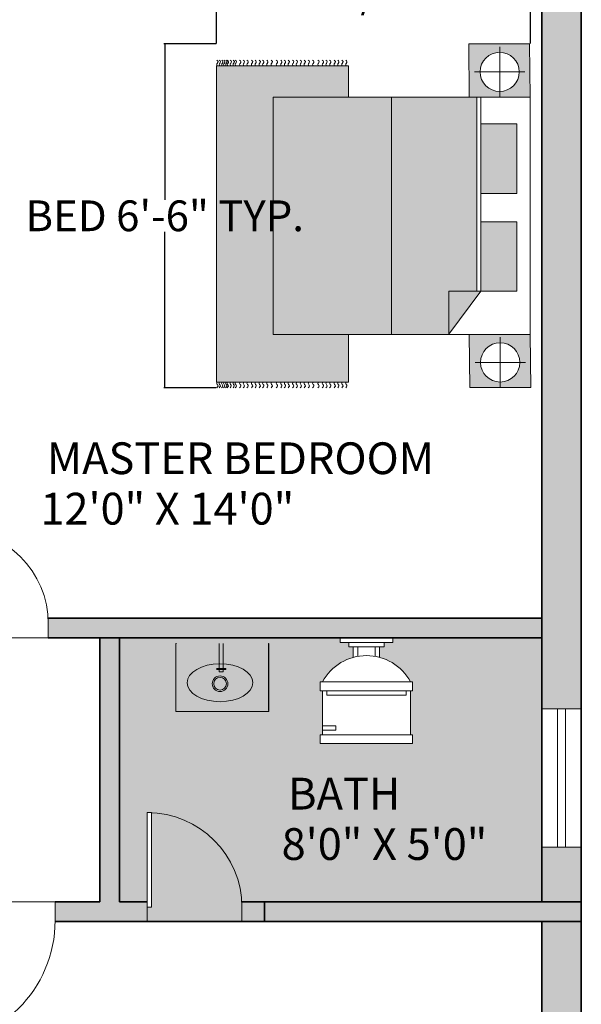
# Model space of a CAD drawing. Units: inches. Extents: x 2167 to 2589, y 1680 to 2489.
# Tile 37 of 38: x 2447 to 2575, y 2143 to 2367. Entities that reach past the tile are written whole.
import ezdxf

# ---------------------------------------------------------------- set-up
doc = ezdxf.new("R2010")
doc.units = ezdxf.units.IN
doc.header["$MEASUREMENT"] = 0
doc.layers.get('0').update_dxf_attribs({"color": 250})
for name, color, linetype, lineweight in [('A-ANNO-DIMS', 2, 'Continuous', 18), ('A-AREA-IDEN', 7, 'Continuous', 18), ('A-DOOR', 4, 'Continuous', 18), ('A-FLOR-FIXT', 8, 'Continuous', 18), ('A-FLOR-TILE-PATT', 252, 'Continuous', 13), ('A-FURN-PATT', 31, 'Continuous', 13), ('A-WALL-PATT', 250, 'Continuous', 13), ('C-PROP', 7, 'Continuous', 35), ('furniture', 34, 'Continuous', 18), ('walls', 7, 'Continuous', 35), ('windows', 141, 'Continuous', 18)]:
    doc.layers.add(name, color=color, linetype=linetype, lineweight=lineweight)
doc.layers.add('A-FLOR-FIXT-PATT', color=7, linetype='Continuous', lineweight=13, true_color=0xebebeb)
doc.styles.get("Standard").update_dxf_attribs({"font": 'arial.ttf'})
doc.dimstyles.get("Standard").update_dxf_attribs({"dimtxt": 7, "dimasz": 0.18, "dimexe": 0.18, "dimexo": 0.0625, "dimgap": 0.09, "dimtad": 0, "dimtih": 1, "dimtoh": 1, "dimdec": 1, "dimzin": 0, "dimdsep": 46, "dimlunit": 3, "dimtxsty": 'Standard', "dimcen": 0.09, "dimadec": 0, "dimazin": 0, "dimtfac": 1, "dimtdec": 1, "dimtofl": 0, "dimtmove": 0, "dimatfit": 3, "dimfxl": 1, "dimtolj": 1, "dimtzin": 0, "dimarcsym": 0})

# ---------------------------------------------------------------- blocks, each defined once
blk = doc.blocks.new('*U2')
for p, q in [((0, 0), (0, -6)), ((40, 0), (40, -6))]:
    blk.add_line(p, q)
blk.add_lwpolyline([(0, 0), (0, 40), (1.75, 40), (1.75, 0)], close=True)
blk.add_arc((0, 0), 40, 0, 90)
blk = doc.blocks.new('*U11')
for p, q in [((-10, 22), (-10, 12)), ((-10, 21), (-7, 21)), ((-7, 21), (-7, 20)), ((10, 12), (10, 22)), ((-7, 20), (-10, 20)), ((10.5, 12), (-10.5, 12)), ((-10.5, 10), (-10.5, 12)), ((9, 13), (-9, 13)), ((-9, 13), (-9, 12)), ((9, 12), (9, 13)), ((10.5, 12), (10.5, 10)), ((10.5, 10), (-10.5, 10)), ((-3, 4.4065), (-3, 2)), ((-2, 2), (-2, 4.1658)), ((2, 4.1658), (2, 2)), ((3, 2), (3, 4.4065)), ((4, 2), (-4, 2)), ((-4, 2), (-4, 1)), ((4, 1), (4, 2))]:
    blk.add_line(p, q)
for points in [[(10.5, 22), (10.5, 24), (-10.5, 24), (-10.5, 22)], [(6, 0), (6, 1), (-6, 1), (-6, 0)]]:
    blk.add_lwpolyline(points, close=True)
blk.add_arc((0, 15.3333), 11.3333, 208.0725, 331.9275)
blk = doc.blocks.new('CARPET')
at = {"layer": 'furniture'}
for p, q in [((-51.53, -98.11), (-51.53, -55.12)), ((-51.53, -55.12), (-41.27, -55.12)), ((36, -55.12), (51.55, -55.12)), ((51.55, -55.12), (51.55, -98.11)), ((51.55, -98.11), (-51.53, -98.11))]:
    blk.add_line(p, q, dxfattribs=at)
for points, knots in [([(-53.37, -55.99), (-53.22, -55.8), (-52.9, -55.41), (-52.34, -55.8), (-51.89, -56.08), (-51.65, -55.91), (-51.53, -55.83)], [0, 0, 0, 0, 0.653278, 1.290138, 1.740457, 2.114451, 2.114451, 2.114451, 2.114451]), ([(-53.37, -57.26), (-53.22, -57.07), (-52.9, -56.67), (-52.34, -57.07), (-51.89, -57.35), (-51.65, -57.17), (-51.53, -57.1)], [0, 0, 0, 0, 0.653278, 1.290138, 1.740457, 2.114451, 2.114451, 2.114451, 2.114451]), ([(53.37, -55.99), (53.22, -55.8), (52.9, -55.41), (52.34, -55.8), (51.89, -56.08), (51.65, -55.91), (51.53, -55.83)], [0, 0, 0, 0, 0.653278, 1.290138, 1.740457, 2.114451, 2.114451, 2.114451, 2.114451]), ([(53.37, -57.26), (53.22, -57.07), (52.9, -56.67), (52.34, -57.07), (51.89, -57.35), (51.65, -57.17), (51.53, -57.1)], [0, 0, 0, 0, 0.653278, 1.290138, 1.740457, 2.114451, 2.114451, 2.114451, 2.114451]), ([(-53.37, -58.59), (-53.22, -58.4), (-52.9, -58.01), (-52.34, -58.4), (-51.89, -58.68), (-51.65, -58.5), (-51.53, -58.43)], [0, 0, 0, 0, 0.653278, 1.290138, 1.740457, 2.114451, 2.114451, 2.114451, 2.114451]), ([(-53.37, -59.78), (-53.22, -59.58), (-52.9, -59.19), (-52.34, -59.58), (-51.89, -59.86), (-51.65, -59.69), (-51.53, -59.61)], [0, 0, 0, 0, 0.653278, 1.290138, 1.740457, 2.114451, 2.114451, 2.114451, 2.114451]), ([(-53.37, -61.22), (-53.22, -61.02), (-52.9, -60.63), (-52.34, -61.02), (-51.89, -61.3), (-51.65, -61.13), (-51.53, -61.05)], [0, 0, 0, 0, 0.653278, 1.290138, 1.740457, 2.114451, 2.114451, 2.114451, 2.114451]), ([(53.37, -58.59), (53.22, -58.4), (52.9, -58.01), (52.34, -58.4), (51.89, -58.68), (51.65, -58.5), (51.53, -58.43)], [0, 0, 0, 0, 0.653278, 1.290138, 1.740457, 2.114451, 2.114451, 2.114451, 2.114451]), ([(53.37, -59.78), (53.22, -59.58), (52.9, -59.19), (52.34, -59.58), (51.89, -59.86), (51.65, -59.69), (51.53, -59.61)], [0, 0, 0, 0, 0.653278, 1.290138, 1.740457, 2.114451, 2.114451, 2.114451, 2.114451]), ([(53.37, -61.22), (53.22, -61.02), (52.9, -60.63), (52.34, -61.02), (51.89, -61.3), (51.65, -61.13), (51.53, -61.05)], [0, 0, 0, 0, 0.653278, 1.290138, 1.740457, 2.114451, 2.114451, 2.114451, 2.114451]), ([(-53.37, -62.44), (-53.22, -62.25), (-52.9, -61.86), (-52.34, -62.25), (-51.89, -62.53), (-51.65, -62.36), (-51.53, -62.28)], [0, 0, 0, 0, 0.653278, 1.290138, 1.740457, 2.114451, 2.114451, 2.114451, 2.114451]), ([(-53.37, -63.63), (-53.22, -63.43), (-52.9, -63.04), (-52.34, -63.43), (-51.89, -63.72), (-51.65, -63.54), (-51.53, -63.46)], [0, 0, 0, 0, 0.653278, 1.290138, 1.740457, 2.114451, 2.114451, 2.114451, 2.114451]), ([(53.37, -62.44), (53.22, -62.25), (52.9, -61.86), (52.34, -62.25), (51.89, -62.53), (51.65, -62.36), (51.53, -62.28)], [0, 0, 0, 0, 0.653278, 1.290138, 1.740457, 2.114451, 2.114451, 2.114451, 2.114451]), ([(53.37, -63.63), (53.22, -63.43), (52.9, -63.04), (52.34, -63.43), (51.89, -63.72), (51.65, -63.54), (51.53, -63.46)], [0, 0, 0, 0, 0.653278, 1.290138, 1.740457, 2.114451, 2.114451, 2.114451, 2.114451]), ([(-53.37, -65.07), (-53.22, -64.87), (-52.9, -64.48), (-52.34, -64.87), (-51.89, -65.15), (-51.65, -64.98), (-51.53, -64.9)], [0, 0, 0, 0, 0.653278, 1.290138, 1.740457, 2.114451, 2.114451, 2.114451, 2.114451]), ([(-53.37, -66.76), (-53.22, -66.56), (-52.9, -66.17), (-52.34, -66.56), (-51.89, -66.84), (-51.65, -66.67), (-51.53, -66.59)], [0, 0, 0, 0, 0.653278, 1.290138, 1.740457, 2.114451, 2.114451, 2.114451, 2.114451]), ([(53.37, -65.07), (53.22, -64.87), (52.9, -64.48), (52.34, -64.87), (51.89, -65.15), (51.65, -64.98), (51.53, -64.9)], [0, 0, 0, 0, 0.653278, 1.290138, 1.740457, 2.114451, 2.114451, 2.114451, 2.114451]), ([(53.37, -66.76), (53.22, -66.56), (52.9, -66.17), (52.34, -66.56), (51.89, -66.84), (51.65, -66.67), (51.53, -66.59)], [0, 0, 0, 0, 0.653278, 1.290138, 1.740457, 2.114451, 2.114451, 2.114451, 2.114451]), ([(-53.37, -68.2), (-53.22, -68), (-52.9, -67.61), (-52.34, -68), (-51.89, -68.28), (-51.65, -68.11), (-51.53, -68.03)], [0, 0, 0, 0, 0.653278, 1.290138, 1.740457, 2.114451, 2.114451, 2.114451, 2.114451]), ([(-53.37, -69.53), (-53.22, -69.33), (-52.9, -68.94), (-52.34, -69.33), (-51.89, -69.61), (-51.65, -69.44), (-51.53, -69.36)], [0, 0, 0, 0, 0.653278, 1.290138, 1.740457, 2.114451, 2.114451, 2.114451, 2.114451]), ([(-53.37, -70.79), (-53.22, -70.6), (-52.9, -70.21), (-52.34, -70.6), (-51.89, -70.88), (-51.65, -70.7), (-51.53, -70.63)], [0, 0, 0, 0, 0.653278, 1.290138, 1.740457, 2.114451, 2.114451, 2.114451, 2.114451]), ([(53.37, -68.2), (53.22, -68), (52.9, -67.61), (52.34, -68), (51.89, -68.28), (51.65, -68.11), (51.53, -68.03)], [0, 0, 0, 0, 0.653278, 1.290138, 1.740457, 2.114451, 2.114451, 2.114451, 2.114451]), ([(53.37, -69.53), (53.22, -69.33), (52.9, -68.94), (52.34, -69.33), (51.89, -69.61), (51.65, -69.44), (51.53, -69.36)], [0, 0, 0, 0, 0.653278, 1.290138, 1.740457, 2.114451, 2.114451, 2.114451, 2.114451]), ([(53.37, -70.79), (53.22, -70.6), (52.9, -70.21), (52.34, -70.6), (51.89, -70.88), (51.65, -70.7), (51.53, -70.63)], [0, 0, 0, 0, 0.653278, 1.290138, 1.740457, 2.114451, 2.114451, 2.114451, 2.114451]), ([(-53.37, -72.12), (-53.22, -71.93), (-52.9, -71.54), (-52.34, -71.93), (-51.89, -72.21), (-51.65, -72.04), (-51.53, -71.96)], [0, 0, 0, 0, 0.653278, 1.290138, 1.740457, 2.114451, 2.114451, 2.114451, 2.114451]), ([(-53.37, -73.31), (-53.22, -73.11), (-52.9, -72.72), (-52.34, -73.11), (-51.89, -73.4), (-51.65, -73.22), (-51.53, -73.14)], [0, 0, 0, 0, 0.653278, 1.290138, 1.740457, 2.114451, 2.114451, 2.114451, 2.114451]), ([(53.37, -72.12), (53.22, -71.93), (52.9, -71.54), (52.34, -71.93), (51.89, -72.21), (51.65, -72.04), (51.53, -71.96)], [0, 0, 0, 0, 0.653278, 1.290138, 1.740457, 2.114451, 2.114451, 2.114451, 2.114451]), ([(53.37, -73.31), (53.22, -73.11), (52.9, -72.72), (52.34, -73.11), (51.89, -73.4), (51.65, -73.22), (51.53, -73.14)], [0, 0, 0, 0, 0.653278, 1.290138, 1.740457, 2.114451, 2.114451, 2.114451, 2.114451]), ([(-53.37, -74.75), (-53.22, -74.55), (-52.9, -74.16), (-52.34, -74.55), (-51.89, -74.83), (-51.65, -74.66), (-51.53, -74.58)], [0, 0, 0, 0, 0.653278, 1.290138, 1.740457, 2.114451, 2.114451, 2.114451, 2.114451]), ([(-53.37, -75.98), (-53.22, -75.78), (-52.9, -75.39), (-52.34, -75.78), (-51.89, -76.06), (-51.65, -75.89), (-51.53, -75.81)], [0, 0, 0, 0, 0.653278, 1.290138, 1.740457, 2.114451, 2.114451, 2.114451, 2.114451]), ([(-53.37, -77.16), (-53.22, -76.96), (-52.9, -76.57), (-52.34, -76.96), (-51.89, -77.25), (-51.65, -77.07), (-51.53, -76.99)], [0, 0, 0, 0, 0.653278, 1.290138, 1.740457, 2.114451, 2.114451, 2.114451, 2.114451]), ([(53.37, -74.75), (53.22, -74.55), (52.9, -74.16), (52.34, -74.55), (51.89, -74.83), (51.65, -74.66), (51.53, -74.58)], [0, 0, 0, 0, 0.653278, 1.290138, 1.740457, 2.114451, 2.114451, 2.114451, 2.114451]), ([(53.37, -75.98), (53.22, -75.78), (52.9, -75.39), (52.34, -75.78), (51.89, -76.06), (51.65, -75.89), (51.53, -75.81)], [0, 0, 0, 0, 0.653278, 1.290138, 1.740457, 2.114451, 2.114451, 2.114451, 2.114451]), ([(53.37, -77.16), (53.22, -76.96), (52.9, -76.57), (52.34, -76.96), (51.89, -77.25), (51.65, -77.07), (51.53, -76.99)], [0, 0, 0, 0, 0.653278, 1.290138, 1.740457, 2.114451, 2.114451, 2.114451, 2.114451]), ([(-53.37, -78.6), (-53.22, -78.4), (-52.9, -78.01), (-52.34, -78.4), (-51.89, -78.68), (-51.65, -78.51), (-51.53, -78.43)], [0, 0, 0, 0, 0.653278, 1.290138, 1.740457, 2.114451, 2.114451, 2.114451, 2.114451]), ([(-53.37, -80.29), (-53.22, -80.09), (-52.9, -79.7), (-52.34, -80.09), (-51.89, -80.37), (-51.65, -80.2), (-51.53, -80.12)], [0, 0, 0, 0, 0.653278, 1.290138, 1.740457, 2.114451, 2.114451, 2.114451, 2.114451]), ([(53.37, -78.6), (53.22, -78.4), (52.9, -78.01), (52.34, -78.4), (51.89, -78.68), (51.65, -78.51), (51.53, -78.43)], [0, 0, 0, 0, 0.653278, 1.290138, 1.740457, 2.114451, 2.114451, 2.114451, 2.114451]), ([(53.37, -80.29), (53.22, -80.09), (52.9, -79.7), (52.34, -80.09), (51.89, -80.37), (51.65, -80.2), (51.53, -80.12)], [0, 0, 0, 0, 0.653278, 1.290138, 1.740457, 2.114451, 2.114451, 2.114451, 2.114451]), ([(-53.37, -81.73), (-53.22, -81.53), (-52.9, -81.14), (-52.34, -81.53), (-51.89, -81.81), (-51.65, -81.64), (-51.53, -81.56)], [0, 0, 0, 0, 0.653278, 1.290138, 1.740457, 2.114451, 2.114451, 2.114451, 2.114451]), ([(-53.37, -83.06), (-53.22, -82.86), (-52.9, -82.47), (-52.34, -82.86), (-51.89, -83.14), (-51.65, -82.97), (-51.53, -82.89)], [0, 0, 0, 0, 0.653278, 1.290138, 1.740457, 2.114451, 2.114451, 2.114451, 2.114451]), ([(53.37, -81.73), (53.22, -81.53), (52.9, -81.14), (52.34, -81.53), (51.89, -81.81), (51.65, -81.64), (51.53, -81.56)], [0, 0, 0, 0, 0.653278, 1.290138, 1.740457, 2.114451, 2.114451, 2.114451, 2.114451]), ([(53.37, -83.06), (53.22, -82.86), (52.9, -82.47), (52.34, -82.86), (51.89, -83.14), (51.65, -82.97), (51.53, -82.89)], [0, 0, 0, 0, 0.653278, 1.290138, 1.740457, 2.114451, 2.114451, 2.114451, 2.114451]), ([(-53.37, -84.18), (-53.22, -83.99), (-52.9, -83.6), (-52.34, -83.99), (-51.89, -84.27), (-51.65, -84.09), (-51.53, -84.02)], [0, 0, 0, 0, 0.653278, 1.290138, 1.740457, 2.114451, 2.114451, 2.114451, 2.114451]), ([(-53.37, -85.51), (-53.22, -85.32), (-52.9, -84.93), (-52.34, -85.32), (-51.89, -85.6), (-51.65, -85.42), (-51.53, -85.35)], [0, 0, 0, 0, 0.653278, 1.290138, 1.740457, 2.114451, 2.114451, 2.114451, 2.114451]), ([(-53.37, -86.7), (-53.22, -86.5), (-52.9, -86.11), (-52.34, -86.5), (-51.89, -86.78), (-51.65, -86.61), (-51.53, -86.53)], [0, 0, 0, 0, 0.653278, 1.290138, 1.740457, 2.114451, 2.114451, 2.114451, 2.114451]), ([(53.37, -84.18), (53.22, -83.99), (52.9, -83.6), (52.34, -83.99), (51.89, -84.27), (51.65, -84.09), (51.53, -84.02)], [0, 0, 0, 0, 0.653278, 1.290138, 1.740457, 2.114451, 2.114451, 2.114451, 2.114451]), ([(53.37, -85.51), (53.22, -85.32), (52.9, -84.93), (52.34, -85.32), (51.89, -85.6), (51.65, -85.42), (51.53, -85.35)], [0, 0, 0, 0, 0.653278, 1.290138, 1.740457, 2.114451, 2.114451, 2.114451, 2.114451]), ([(53.37, -86.7), (53.22, -86.5), (52.9, -86.11), (52.34, -86.5), (51.89, -86.78), (51.65, -86.61), (51.53, -86.53)], [0, 0, 0, 0, 0.653278, 1.290138, 1.740457, 2.114451, 2.114451, 2.114451, 2.114451]), ([(-53.37, -88.14), (-53.22, -87.94), (-52.9, -87.55), (-52.34, -87.94), (-51.89, -88.22), (-51.65, -88.05), (-51.53, -87.97)], [0, 0, 0, 0, 0.653278, 1.290138, 1.740457, 2.114451, 2.114451, 2.114451, 2.114451]), ([(-53.37, -89.36), (-53.22, -89.17), (-52.9, -88.78), (-52.34, -89.17), (-51.89, -89.45), (-51.65, -89.28), (-51.53, -89.2)], [0, 0, 0, 0, 0.653278, 1.290138, 1.740457, 2.114451, 2.114451, 2.114451, 2.114451]), ([(53.37, -88.14), (53.22, -87.94), (52.9, -87.55), (52.34, -87.94), (51.89, -88.22), (51.65, -88.05), (51.53, -87.97)], [0, 0, 0, 0, 0.653278, 1.290138, 1.740457, 2.114451, 2.114451, 2.114451, 2.114451]), ([(53.37, -89.36), (53.22, -89.17), (52.9, -88.78), (52.34, -89.17), (51.89, -89.45), (51.65, -89.28), (51.53, -89.2)], [0, 0, 0, 0, 0.653278, 1.290138, 1.740457, 2.114451, 2.114451, 2.114451, 2.114451]), ([(-53.37, -90.55), (-53.22, -90.35), (-52.9, -89.96), (-52.34, -90.35), (-51.89, -90.64), (-51.65, -90.46), (-51.53, -90.38)], [0, 0, 0, 0, 0.653278, 1.290138, 1.740457, 2.114451, 2.114451, 2.114451, 2.114451]), ([(-53.37, -91.99), (-53.22, -91.79), (-52.9, -91.4), (-52.34, -91.79), (-51.89, -92.07), (-51.65, -91.9), (-51.53, -91.82)], [0, 0, 0, 0, 0.653278, 1.290138, 1.740457, 2.114451, 2.114451, 2.114451, 2.114451]), ([(-53.37, -92.69), (-53.22, -92.48), (-52.9, -92.08), (-52.35, -92.49), (-51.89, -92.77), (-51.65, -92.6), (-51.53, -92.52)], [0, 0, 0, 0, 0.663904, 1.307406, 1.757725, 2.131719, 2.131719, 2.131719, 2.131719]), ([(53.37, -90.55), (53.22, -90.35), (52.9, -89.96), (52.34, -90.35), (51.9, -90.63), (51.66, -90.47), (51.55, -90.4)], [0, 0, 0, 0, 0.653278, 1.290138, 1.740457, 2.0926, 2.0926, 2.0926, 2.0926]), ([(53.37, -91.99), (53.22, -91.79), (52.9, -91.4), (52.34, -91.79), (51.9, -92.07), (51.66, -91.91), (51.55, -91.83)], [0, 0, 0, 0, 0.653278, 1.290138, 1.740457, 2.0926, 2.0926, 2.0926, 2.0926]), ([(53.37, -92.69), (53.22, -92.49), (52.9, -92.09), (52.34, -92.49), (51.9, -92.77), (51.66, -92.61), (51.55, -92.53)], [0, 0, 0, 0, 0.656792, 1.295826, 1.746145, 2.098292, 2.098292, 2.098292, 2.098292]), ([(-53.37, -93.61), (-53.22, -93.42), (-52.9, -93.03), (-52.34, -93.42), (-51.89, -93.7), (-51.65, -93.52), (-51.53, -93.45)], [0, 0, 0, 0, 0.653278, 1.290138, 1.740457, 2.114451, 2.114451, 2.114451, 2.114451]), ([(-53.37, -94.55), (-53.22, -94.35), (-52.9, -93.96), (-52.34, -94.35), (-51.89, -94.63), (-51.65, -94.46), (-51.53, -94.38)], [0, 0, 0, 0, 0.653278, 1.290138, 1.740457, 2.114451, 2.114451, 2.114451, 2.114451]), ([(-53.37, -95.05), (-53.22, -94.85), (-52.9, -94.46), (-52.34, -94.85), (-51.89, -95.14), (-51.65, -94.96), (-51.53, -94.88)], [0, 0, 0, 0, 0.653278, 1.290138, 1.740457, 2.114451, 2.114451, 2.114451, 2.114451]), ([(-53.37, -95.73), (-53.22, -95.54), (-52.9, -95.15), (-52.34, -95.54), (-51.89, -95.82), (-51.65, -95.65), (-51.53, -95.57)], [0, 0, 0, 0, 0.653278, 1.290138, 1.740457, 2.114451, 2.114451, 2.114451, 2.114451]), ([(-53.37, -96.38), (-53.22, -96.18), (-52.9, -95.79), (-52.34, -96.18), (-51.89, -96.47), (-51.65, -96.29), (-51.53, -96.21)], [0, 0, 0, 0, 0.653278, 1.290138, 1.740457, 2.114451, 2.114451, 2.114451, 2.114451]), ([(53.37, -95.78), (53.22, -95.58), (52.9, -95.19), (52.34, -95.58), (51.89, -95.86), (51.65, -95.69), (51.53, -95.61)], [0, 0, 0, 0, 0.653278, 1.290138, 1.740457, 2.114451, 2.114451, 2.114451, 2.114451]), ([(53.37, -96.43), (53.22, -96.23), (52.9, -95.84), (52.34, -96.23), (51.89, -96.51), (51.65, -96.34), (51.53, -96.26)], [0, 0, 0, 0, 0.653278, 1.290138, 1.740457, 2.114451, 2.114451, 2.114451, 2.114451]), ([(53.37, -93.66), (53.22, -93.46), (52.9, -93.07), (52.34, -93.46), (51.9, -93.74), (51.66, -93.58), (51.55, -93.5)], [0, 0, 0, 0, 0.653278, 1.290138, 1.740457, 2.0926, 2.0926, 2.0926, 2.0926]), ([(53.37, -94.59), (53.22, -94.4), (52.9, -94.01), (52.34, -94.4), (51.9, -94.68), (51.66, -94.51), (51.55, -94.44)], [0, 0, 0, 0, 0.653278, 1.290138, 1.740457, 2.0926, 2.0926, 2.0926, 2.0926]), ([(53.37, -95.1), (53.22, -94.9), (52.9, -94.51), (52.34, -94.9), (51.9, -95.18), (51.66, -95.02), (51.55, -94.94)], [0, 0, 0, 0, 0.653278, 1.290138, 1.740457, 2.0926, 2.0926, 2.0926, 2.0926]), ([(-53.37, -97.17), (-53.22, -96.98), (-52.9, -96.59), (-52.34, -96.98), (-51.89, -97.26), (-51.65, -97.08), (-51.53, -97.01)], [0, 0, 0, 0, 0.653278, 1.290138, 1.740457, 2.114451, 2.114451, 2.114451, 2.114451]), ([(-53.37, -97.99), (-53.22, -97.79), (-52.9, -97.4), (-52.34, -97.79), (-51.89, -98.08), (-51.65, -97.9), (-51.53, -97.82)], [0, 0, 0, 0, 0.653278, 1.290138, 1.740457, 2.114451, 2.114451, 2.114451, 2.114451]), ([(53.37, -97.22), (53.22, -97.02), (52.9, -96.63), (52.34, -97.02), (51.89, -97.3), (51.65, -97.13), (51.53, -97.05)], [0, 0, 0, 0, 0.653278, 1.290138, 1.740457, 2.114451, 2.114451, 2.114451, 2.114451]), ([(53.37, -97.99), (53.22, -97.79), (52.9, -97.4), (52.34, -97.79), (51.89, -98.08), (51.65, -97.9), (51.53, -97.82)], [0, 0, 0, 0, 0.653278, 1.290138, 1.740457, 2.114451, 2.114451, 2.114451, 2.114451])]:
    blk.add_open_spline(points, degree=3, knots=knots, dxfattribs=at)
blk = doc.blocks.new('A$C58D270C6')
at = {"layer": 'furniture'}
for p, q in [((9.09, 124.13), (9.09, 108.87)), ((1.46, 116.5), (16.73, 116.5)), ((14.97, 94.84), (24.62, 107.92)), ((24.62, 94.93), (24.62, 107.92)), ((42.08, 108), (42.08, 36)), ((14.97, 94.93), (24.62, 94.93)), ((14.97, 94.84), (14.97, 36)), ((16.22, 94.93), (16.22, 36)), ((9.25, 36), (9.25, 20.74)), ((1.62, 28.37), (16.88, 28.37))]:
    blk.add_line(p, q, dxfattribs=at)
for points in [[(18.5, 108), (18.34, 124.13), (-0.16, 124.13), (0, 108)], [(0, 108), (77.91, 108), (77.91, 36), (0, 36)], [(4.09, 94.93), (14.97, 94.93), (14.97, 73.83), (4.09, 73.83)], [(4.09, 65.23), (14.97, 65.23), (14.97, 44.13), (4.09, 44.13)], [(18.65, 19.87), (18.5, 36), (0, 36), (0.16, 19.87)]]:
    blk.add_lwpolyline(points, close=True, dxfattribs=at)
for centre in [(9.09, 116.5), (9.25, 28.37)]:
    blk.add_circle(centre, 5.95, dxfattribs=at)
at = {"layer": 'furniture', "xscale": 0.9312884925094044, "yscale": 0.9312884925094044, "zscale": 0.9312884925094044, "rotation": 90}
blk.add_blockref('CARPET', (3.79, 74.47), dxfattribs=at)
blk = doc.blocks.new('LAV-OVAL-WITH-TAP')
for p, q in [((6.14, 5.63), (6.14, 5.92)), ((6.14, 5.92), (8.26, 5.92)), ((8.26, 5.63), (6.14, 5.63)), ((7.69, 6.42), (6.74, 6.42)), ((6.74, 6.42), (6.74, 0)), ((7.69, 6.42), (7.69, 0))]:
    blk.add_line(p, q)
for radius in [1.79, 1.79, 1.43, 1.43, 1.43, 1.43]:
    blk.add_circle((7.46, 9.13), radius)
blk.add_ellipse((7.48, 8.9), major_axis=(7.48, 0.02), ratio=0.576535)
blk = doc.blocks.new('*D43')
at = {"layer": 'A-ANNO-DIMS', "color": 0, "lineweight": -2, "transparency": 16777216}
for p, q in [((2491.99, 2361.37), (2480.13, 2361.37)), ((2480.31, 2361.19), (2480.31, 2325.91)), ((2480.31, 2283.31), (2480.31, 2318.59)), ((2491.99, 2283.13), (2480.13, 2283.13))]:
    blk.add_line(p, q, dxfattribs=at)
at = {"layer": 'A-ANNO-DIMS', "color": 0, "transparency": 16777216}
for points in [[(2480.28, 2361.19), (2480.34, 2361.19), (2480.31, 2361.37)], [(2480.28, 2283.31), (2480.34, 2283.31), (2480.31, 2283.13)]]:
    blk.add_solid(points, dxfattribs=at)
at = {"layer": 'Defpoints', "color": 0, "transparency": 16777216}
for p in [(2492.05, 2361.37), (2480.31, 2283.13), (2492.05, 2283.13)]:
    blk.add_point(p, dxfattribs=at)
at = {"layer": 'A-ANNO-DIMS', "color": 0, "transparency": 16777216, "insert": (2480.31, 2322.25), "char_height": 7, "attachment_point": 5}
blk.add_mtext('\\A1;BED 6\'-6" TYP.', dxfattribs=at)
blk = doc.blocks.new('*D44')
at = {"layer": 'A-ANNO-DIMS', "color": 0, "lineweight": -2, "transparency": 16777216}
for p, q in [((2492.05, 2361.43), (2492.05, 2373.28)), ((2492.23, 2373.1), (2495.49, 2373.1)), ((2563.35, 2373.1), (2560.09, 2373.1)), ((2563.53, 2361.43), (2563.53, 2373.28))]:
    blk.add_line(p, q, dxfattribs=at)
at = {"layer": 'A-ANNO-DIMS', "color": 0, "transparency": 16777216}
for points in [[(2492.23, 2373.13), (2492.23, 2373.07), (2492.05, 2373.1)], [(2563.35, 2373.13), (2563.35, 2373.07), (2563.53, 2373.1)]]:
    blk.add_solid(points, dxfattribs=at)
at = {"layer": 'Defpoints', "color": 0, "transparency": 16777216}
for p in [(2492.05, 2373.1), (2492.05, 2361.37), (2563.53, 2361.37)]:
    blk.add_point(p, dxfattribs=at)
at = {"layer": 'A-ANNO-DIMS', "color": 0, "transparency": 16777216, "insert": (2527.79, 2373.1), "char_height": 7, "attachment_point": 5}
blk.add_mtext('\\A1;5\'-11 1/2" TYP.', dxfattribs=at)

msp = doc.modelspace()

# ---------------------------------------------------------------- hatches: boundary and pattern name
at = {"layer": 'A-FLOR-FIXT-PATT'}
h = msp.add_hatch(color=256, dxfattribs=at)
h.dxf.hatch_style = 1
edge = h.paths.add_edge_path()
edge.add_line((2483, 2209.66), (2503.9, 2209.66))
edge.add_line((2503.9, 2209.66), (2503.9, 2224.91))
edge.add_line((2503.9, 2224.91), (2493.61, 2224.91))
edge.add_line((2493.61, 2224.91), (2493.61, 2220.31))
edge.add_ellipse((2492.87, 2216.02), major_axis=(-7.48, -0.02), ratio=0.576535, start_angle=272.6137, end_angle=620.1108, ccw=False)
edge.add_line((2492.66, 2220.33), (2492.66, 2224.91))
edge.add_line((2492.66, 2224.91), (2483, 2224.91))
edge.add_line((2483, 2224.91), (2483, 2209.66))
h = msp.add_hatch(color=256, dxfattribs=at)
h.dxf.hatch_style = 1
edge = h.paths.add_edge_path()
edge.add_ellipse((2492.87, 2216.02), major_axis=(-7.48, -0.02), ratio=0.576535, start_angle=272.6137, end_angle=260.1108)
edge.add_line((2493.61, 2220.31), (2493.61, 2219.29))
edge.add_line((2493.61, 2219.29), (2494.21, 2219.29))
edge.add_line((2494.21, 2219.29), (2494.21, 2218.99))
edge.add_line((2494.21, 2218.99), (2493.61, 2218.99))
edge.add_line((2493.61, 2218.99), (2493.61, 2218.49))
edge.add_line((2493.61, 2218.49), (2492.66, 2218.49))
edge.add_line((2492.66, 2218.49), (2492.66, 2220.33))
h.paths.add_polyline_path([(2491.1, 2215.78, -1), (2494.67, 2215.78, -1)], flags=16)
h.paths.add_polyline_path([(2494.31, 2215.78, -1), (2491.46, 2215.78, -1)], flags=0)
h.paths.add_polyline_path([(2491.46, 2215.78, 1), (2494.31, 2215.78, 1)], flags=0)
edge = h.paths.add_edge_path()
edge.add_line((2492.66, 2219.29), (2493.61, 2219.29))
edge.add_line((2493.61, 2219.29), (2493.61, 2220.31))
edge.add_ellipse((2492.87, 2216.02), major_axis=(-7.48, -0.02), ratio=0.576535, start_angle=260.1108, end_angle=272.6137)
edge.add_line((2492.66, 2220.33), (2492.66, 2219.29))
h.paths.add_polyline_path([(2492.66, 2218.49), (2493.61, 2218.49), (2493.61, 2218.99), (2492.66, 2218.99)], flags=17)
h.paths.add_polyline_path([(2492.66, 2218.99), (2493.61, 2218.99), (2493.61, 2219.29), (2492.66, 2219.29)], flags=17)
h.paths.add_polyline_path([(2493.61, 2218.99), (2494.21, 2218.99), (2494.21, 2219.29), (2493.61, 2219.29)], flags=17)
edge = h.paths.add_edge_path()
edge.add_ellipse((2492.87, 2216.02), major_axis=(-7.48, -0.02), ratio=0.576535, start_angle=260.1108, end_angle=272.6137, ccw=False)
edge.add_line((2493.61, 2220.31), (2493.61, 2224.91))
edge.add_line((2493.61, 2224.91), (2492.66, 2224.91))
edge.add_line((2492.66, 2224.91), (2492.66, 2220.33))
h = msp.add_hatch(color=256, dxfattribs=at)
h.dxf.hatch_style = 1
h.paths.add_polyline_path([(2494.31, 2215.78, 1), (2491.46, 2215.78, 1)], flags=0)
h.paths.add_polyline_path([(2494.67, 2215.78, 1), (2491.1, 2215.78, 1)])
h.paths.add_polyline_path([(2494.31, 2215.78, -1), (2491.46, 2215.78, -1)], flags=16)
h = msp.add_hatch(color=256, dxfattribs=at)
h.dxf.hatch_style = 1
h.paths.add_polyline_path([(2494.31, 2215.78, 1), (2491.46, 2215.78, 1)])
at = {"layer": 'A-FLOR-TILE-PATT'}
h = msp.add_hatch(dxfattribs=at)
h.set_pattern_fill('ANGLE', color=256, scale=5)
h.set_pattern_definition([(0, (0, 0), (0, 1.375), [1, -0.375]), (90, (0, 0), (-1.375, 1e-16), [1, -0.375])])
h.paths.add_polyline_path([(2566.05, 2226.19), (2532.19, 2226.19), (2532.19, 2225.19), (2530.19, 2225.19), (2530.19, 2224.19), (2529.19, 2224.19), (2529.19, 2221.79, -0.206081), (2536.19, 2216.19), (2536.69, 2216.19), (2536.69, 2214.19), (2536.19, 2214.19), (2536.19, 2204.19), (2536.69, 2204.19), (2536.69, 2202.19), (2515.69, 2202.19), (2515.69, 2204.19), (2516.19, 2204.19), (2516.19, 2214.19), (2515.69, 2214.19), (2515.69, 2216.19), (2516.19, 2216.19, -0.206081), (2523.19, 2221.79), (2523.19, 2224.19), (2522.19, 2224.19), (2522.19, 2225.19), (2520.19, 2225.19), (2520.19, 2226.19), (2470.05, 2226.19), (2470.05, 2166.19), (2476.35, 2166.19), (2476.35, 2186.45), (2477.29, 2186.45), (2477.29, 2186.43, -0.38441), (2497.84, 2166.19), (2566.05, 2166.19)])
h.paths.add_polyline_path([(2504.02, 2209.46), (2504.02, 2224.91), (2503.9, 2224.91), (2503.9, 2209.66)], flags=16)
edge = h.paths.add_edge_path(flags=16)
edge.add_ellipse((2492.87, 2216.02), major_axis=(-7.48, -0.02), ratio=0.576535, start_angle=272.6137, end_angle=620.1108, ccw=False)
edge.add_ellipse((2492.87, 2216.02), major_axis=(-7.48, -0.02), ratio=0.576535, start_angle=260.1108, end_angle=272.6137, ccw=False)
h.paths.add_polyline_path([(2491.1, 2215.78, -1), (2494.67, 2215.78, -1)], flags=0)
h.paths.add_polyline_path([(2494.31, 2215.78, -1), (2491.46, 2215.78, -1)], flags=0)
h.paths.add_polyline_path([(2494.21, 2218.99), (2493.61, 2218.99), (2493.61, 2218.49), (2492.66, 2218.49), (2492.66, 2219.29), (2494.21, 2219.29)], flags=0)
h.paths.add_polyline_path([(2477.29, 2186.43), (2477.29, 2164.92), (2476.35, 2164.92), (2476.35, 2161.69), (2497.88, 2161.69), (2497.88, 2164.92, 0.401453)])
at = {"layer": 'A-FURN-PATT'}
h = msp.add_hatch(color=256, dxfattribs=at)
h.dxf.hatch_style = 1
h.paths.add_polyline_path([(2552.01, 2354.99, -1), (2560.95, 2354.99, -0.414214), (2556.48, 2350.53), (2556.48, 2349.27), (2563.42, 2349.27), (2563.3, 2361.37), (2549.43, 2361.37), (2549.54, 2349.27), (2556.48, 2349.27), (2556.48, 2350.53, -0.414214)])
h.paths.add_polyline_path([(2561.06, 2288.89, -0.414214), (2556.6, 2284.43), (2556.6, 2283.17), (2563.53, 2283.17), (2563.42, 2295.27), (2549.54, 2295.27), (2549.66, 2283.17), (2556.6, 2283.17), (2556.6, 2284.43, -0.414214), (2552.13, 2288.89, -1)])
h.paths.add_polyline_path([(2552.14, 2305.07), (2544.95, 2305.07), (2544.95, 2295.33)])
h = msp.add_hatch(color=256, dxfattribs=at)
h.dxf.hatch_style = 1
h.paths.add_polyline_path([(2504.99, 2349.27), (2522.07, 2349.27), (2522.07, 2356.41), (2492.05, 2356.41), (2492.05, 2284.4), (2522.07, 2284.4), (2522.07, 2295.27), (2504.99, 2295.27)])
h.paths.add_polyline_path([(2531.86, 2349.27), (2504.99, 2349.27), (2504.99, 2295.27), (2531.86, 2295.27)])
h = msp.add_hatch(color=256, dxfattribs=at)
h.dxf.hatch_style = 1
h.paths.add_polyline_path([(2551.25, 2349.27), (2531.86, 2349.27), (2531.86, 2295.27), (2544.91, 2295.27), (2544.95, 2295.33), (2544.95, 2305.07), (2551.25, 2305.07)])
h = msp.add_hatch(color=256, dxfattribs=at)
h.dxf.hatch_style = 1
h.paths.add_polyline_path([(2560.35, 2343.17), (2552.19, 2343.17), (2552.19, 2327.35), (2560.35, 2327.35)])
h.paths.add_polyline_path([(2560.35, 2320.89), (2552.19, 2320.89), (2552.19, 2305.07), (2560.35, 2305.07)])
at = {"layer": 'A-WALL-PATT'}
h = msp.add_hatch(color=256, dxfattribs=at)
h.dxf.hatch_style = 1
h.paths.add_polyline_path([(2575.05, 2407.69), (2518.45, 2407.69), (2518.45, 2398.69), (2566.05, 2398.69), (2566.05, 2210.05), (2568.65, 2210.05), (2575.05, 2210.05)])
h.paths.add_polyline_path([(2503.01, 2166.19), (2497.84, 2166.19, -0.014764), (2497.88, 2164.92), (2497.88, 2161.69), (2503.01, 2161.69)])
h = msp.add_hatch(color=256, dxfattribs=at)
h.dxf.hatch_style = 1
h.paths.add_polyline_path([(2575.05, 2029.69), (2422.05, 2029.69), (2422.05, 2161.69), (2427.02, 2161.69), (2427.02, 2161.94), (2427.02, 2166.19), (2417.55, 2166.19), (2417.55, 2025.19), (2575.05, 2025.19)])
h.paths.add_polyline_path([(2575.05, 2166.19), (2503.01, 2166.19), (2503.01, 2161.69), (2575.05, 2161.69)], flags=17)
h.paths.add_polyline_path([(2575.05, 2161.69), (2566.05, 2161.69), (2566.05, 2029.69), (2575.05, 2029.69)], flags=17)
h.paths.add_polyline_path([(2575.05, 2025.19), (2566.05, 2025.19), (2566.05, 1869.19), (2575.05, 1869.19)])
h.paths.add_polyline_path([(2575.05, 1869.19), (2566.05, 1869.19), (2447.7, 1869.19, -0.014764), (2447.74, 1867.92), (2447.74, 1864.69), (2575.05, 1864.69)])
h.paths.add_polyline_path([(2530.05, 1864.69), (2525.55, 1864.69), (2525.55, 1816.69), (2452.05, 1816.69), (2452.05, 1812.19), (2530.05, 1812.19)])
h.paths.add_polyline_path([(2455.04, 1830.65), (2452.05, 1830.65), (2452.05, 1816.69), (2455.04, 1816.69)], flags=17)
h.paths.add_polyline_path([(2575.05, 1864.69), (2566.05, 1864.69), (2566.05, 1788.19), (2456.1, 1788.19), (2456.1, 1783.94, -0.042065), (2455.7, 1779.19), (2527.68, 1779.19), (2527.68, 1687.69), (2532.18, 1687.69), (2532.18, 1779.19), (2575.05, 1779.19)])
h.paths.add_polyline_path([(2421.87, 1696.69), (2416.11, 1696.69), (2416.11, 1687.69), (2421.87, 1687.69)])
h.paths.add_polyline_path([(2375.61, 1696.69), (2369.84, 1696.69), (2369.84, 1687.69), (2375.61, 1687.69)])
h.paths.add_polyline_path([(2425.05, 2245.69), (2420.55, 2245.69), (2420.55, 2226.19), (2432.29, 2226.19), (2432.29, 2229.42), (2432.29, 2230.69), (2425.05, 2230.69)])
h.paths.add_polyline_path([(2224.05, 2151.19), (2318.55, 2151.19), (2318.55, 2177.3), (2314.78, 2177.3, -0.007324), (2314.05, 2177.32), (2314.05, 2155.69), (2224.05, 2155.69), (2224.05, 2157.46), (2215.05, 2157.46), (2215.05, 2103.59), (2218.97, 2103.59), (2224.05, 2103.59)])
h = msp.add_hatch(color=256, dxfattribs=at)
h.dxf.hatch_style = 1
h.paths.add_polyline_path([(2566.05, 2230.69), (2453.78, 2230.69, -0.014764), (2453.82, 2229.42), (2453.82, 2226.19), (2566.05, 2226.19)])
h.paths.add_polyline_path([(2470.05, 2226.19), (2465.55, 2226.19), (2465.55, 2166.19), (2455.38, 2166.19), (2455.38, 2161.69), (2476.35, 2161.69), (2476.35, 2164.92), (2476.35, 2166.19), (2470.05, 2166.19)])
h = msp.add_hatch(color=256, dxfattribs=at)
h.dxf.hatch_style = 1
h.paths.add_polyline_path([(2575.05, 2178.63), (2566.05, 2178.63), (2566.05, 2166.19), (2575.05, 2166.19)])

# ---------------------------------------------------------------- linework, layer by layer
at = {"layer": 'A-DOOR'}
for p, q in [((2432.29, 2226.19), (2453.82, 2226.19)), ((2427.02, 2166.19), (2455.38, 2166.19))]:
    msp.add_line(p, q, dxfattribs=at)
at = {"layer": 'A-FLOR-FIXT'}
for p, q in [((2482.97, 2224.9), (2482.86, 2224.9)), ((2482.86, 2224.9), (2482.86, 2209.46)), ((2503.9, 2209.66), (2503.9, 2224.91)), ((2504.02, 2224.91), (2503.9, 2224.91)), ((2504.02, 2209.46), (2504.02, 2224.91)), ((2482.86, 2209.46), (2504.02, 2209.46))]:
    msp.add_line(p, q, dxfattribs=at)
at = {"layer": 'C-PROP'}
msp.add_line((2575.05, 2407.69), (2575.05, 1687.69), dxfattribs=at)
at = {"layer": 'walls'}
for p, q in [((2566.05, 2398.69), (2566.05, 2166.19)), ((2453.78, 2230.69), (2566.05, 2230.69)), ((2453.82, 2226.19), (2566.05, 2226.19)), ((2465.55, 2226.19), (2465.55, 2166.19)), ((2470.05, 2226.19), (2470.05, 2166.19)), ((2455.38, 2166.19), (2465.55, 2166.19)), ((2470.05, 2166.19), (2476.35, 2166.19)), ((2497.84, 2166.19), (2575.05, 2166.19)), ((2503.01, 2166.19), (2503.01, 2161.69)), ((2455.38, 2161.69), (2575.05, 2161.69)), ((2566.05, 2161.69), (2566.05, 2029.69))]:
    msp.add_line(p, q, dxfattribs=at)
at = {"layer": 'windows'}
for p, q in [((2566.05, 2210.05), (2575.05, 2210.05)), ((2566.05, 2178.63), (2566.05, 2210.05)), ((2566.05, 2210.05), (2568.65, 2210.05)), ((2569.6, 2210.05), (2569.6, 2178.63)), ((2571.49, 2178.63), (2571.49, 2210.05)), ((2575.05, 2210.05), (2575.05, 2178.63)), ((2575.05, 2178.63), (2566.05, 2178.63)), ((2568.65, 2178.63), (2570.55, 2178.63))]:
    msp.add_line(p, q, dxfattribs=at)

# ---------------------------------------------------------------- block references
at = {"layer": 'A-DOOR', "xscale": 0.5382298898187942, "yscale": 0.5382298898187942, "zscale": 0.5382298898187942}
for p in [(2432.29, 2229.42), (2476.35, 2164.92)]:
    msp.add_blockref('*U2', p, dxfattribs=at)
at = {"layer": 'A-DOOR', "xscale": -0.7089553820317277, "yscale": 0.7089553820317277, "zscale": 0.7089553820317277, "rotation": 180}
msp.add_blockref('*U2', (2427.02, 2161.94), dxfattribs=at)
at = {"layer": 'A-FLOR-FIXT', "rotation": 180}
msp.add_blockref('LAV-OVAL-WITH-TAP', (2500.35, 2224.91), dxfattribs=at)
at = {"layer": 'A-FLOR-FIXT', "xscale": -1, "rotation": 180}
msp.add_blockref('*U11', (2526.19, 2226.19), dxfattribs=at)
at = {"layer": 'furniture', "xscale": 0.7500000390647866, "yscale": 0.7500000390647866, "zscale": 0.7500000390647866, "rotation": 180}
msp.add_blockref('A$C58D270C6', (2563.42, 2376.27), dxfattribs=at)

# ---------------------------------------------------------------- texts
at = {"layer": 'A-AREA-IDEN'}
for s, height, p in [('MASTER BEDROOM', 7.2272, (2453.51, 2263.47)), ('12\'0" X 14\'0"', 7.2272, (2452.03, 2252)), ('BATH', 7.227, (2508.37, 2187.16)), ('8\'0" X 5\'0"', 7.2272, (2506.89, 2175.69))]:
    msp.add_text(s, height=height, dxfattribs=at).set_placement(p)

# ---------------------------------------------------------------- dimensions: what is measured, and where the dimension line sits
at = {"layer": 'A-ANNO-DIMS'}
for base, p1, p2, angle, text, picture, middle in [((2492.05, 2373.1), (2563.53, 2361.37), (2492.05, 2361.37), 180, '<> TYP.', '*D44', (2527.79, 2373.1)), ((2480.31, 2283.13), (2492.05, 2361.37), (2492.05, 2283.13), 270, 'BED <> TYP.', '*D43', (2480.31, 2322.25))]:
    dim = msp.add_linear_dim(base=base, p1=p1, p2=p2, angle=angle, text=text, dimstyle='Standard', override={"dimdec": 1, "dimlfac": 1, "dimrnd": 0, "dimzin": 1, "dimdsep": 46, "dimlunit": 4, "dimfrac": 2}, dxfattribs=at)
    dim.commit()
    dim.dimension.update_dxf_attribs({"geometry": picture, "text_midpoint": middle})

doc.saveas('drawing.dxf')
